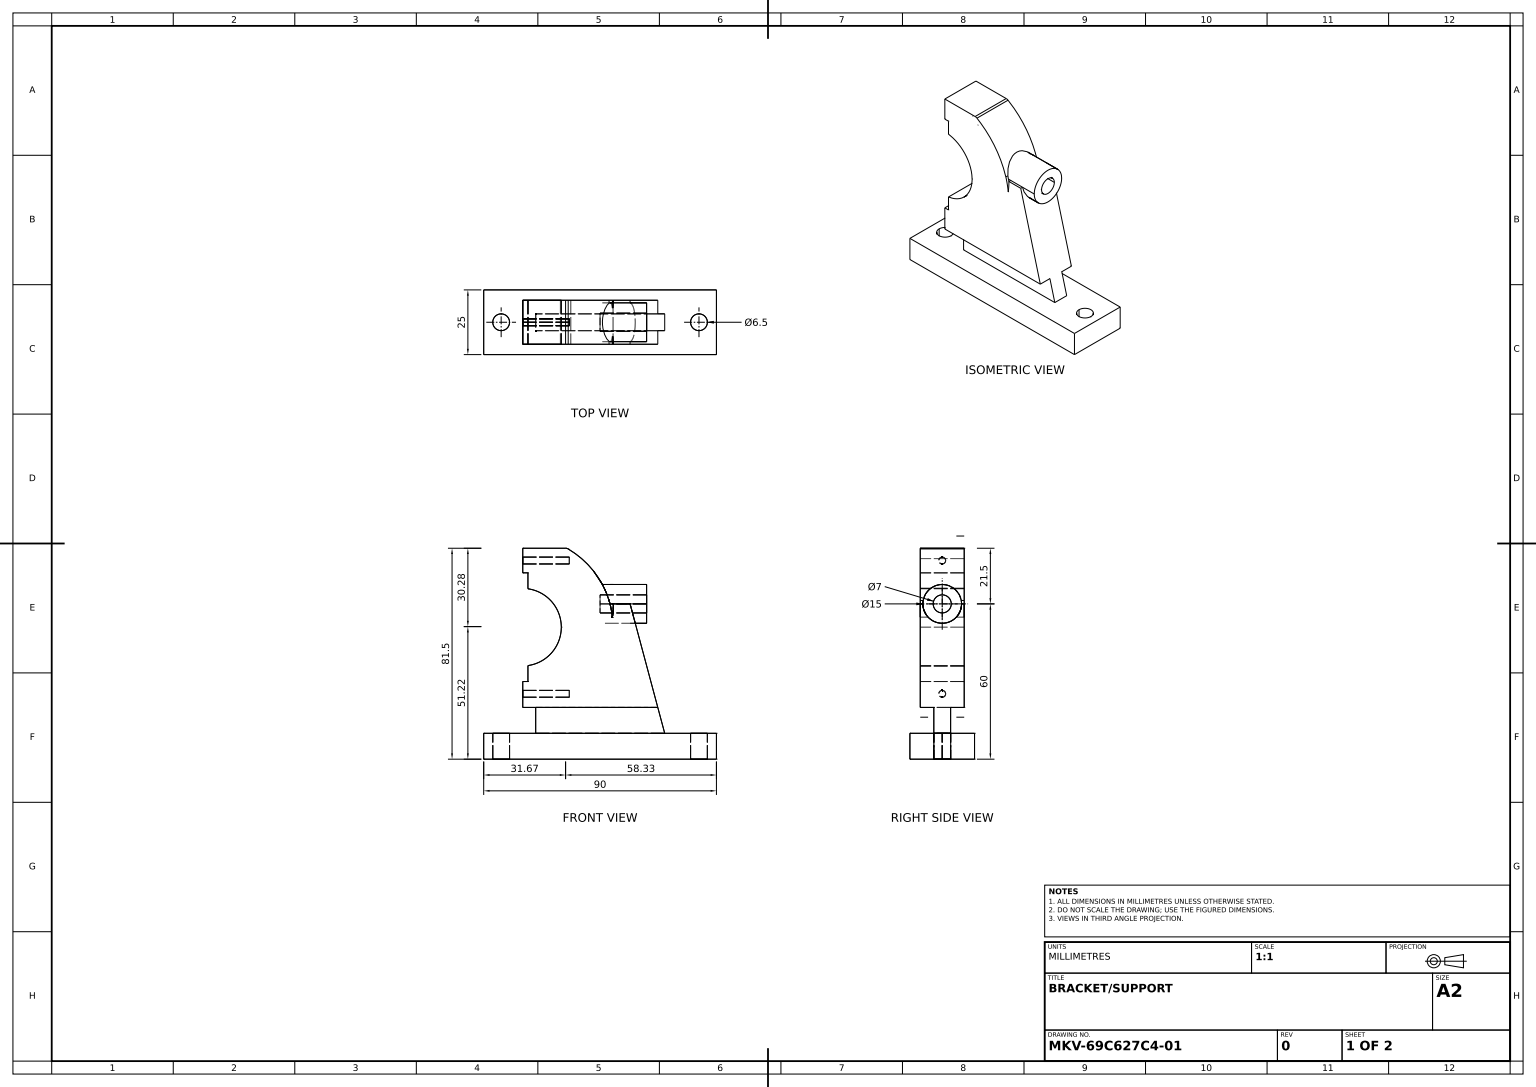
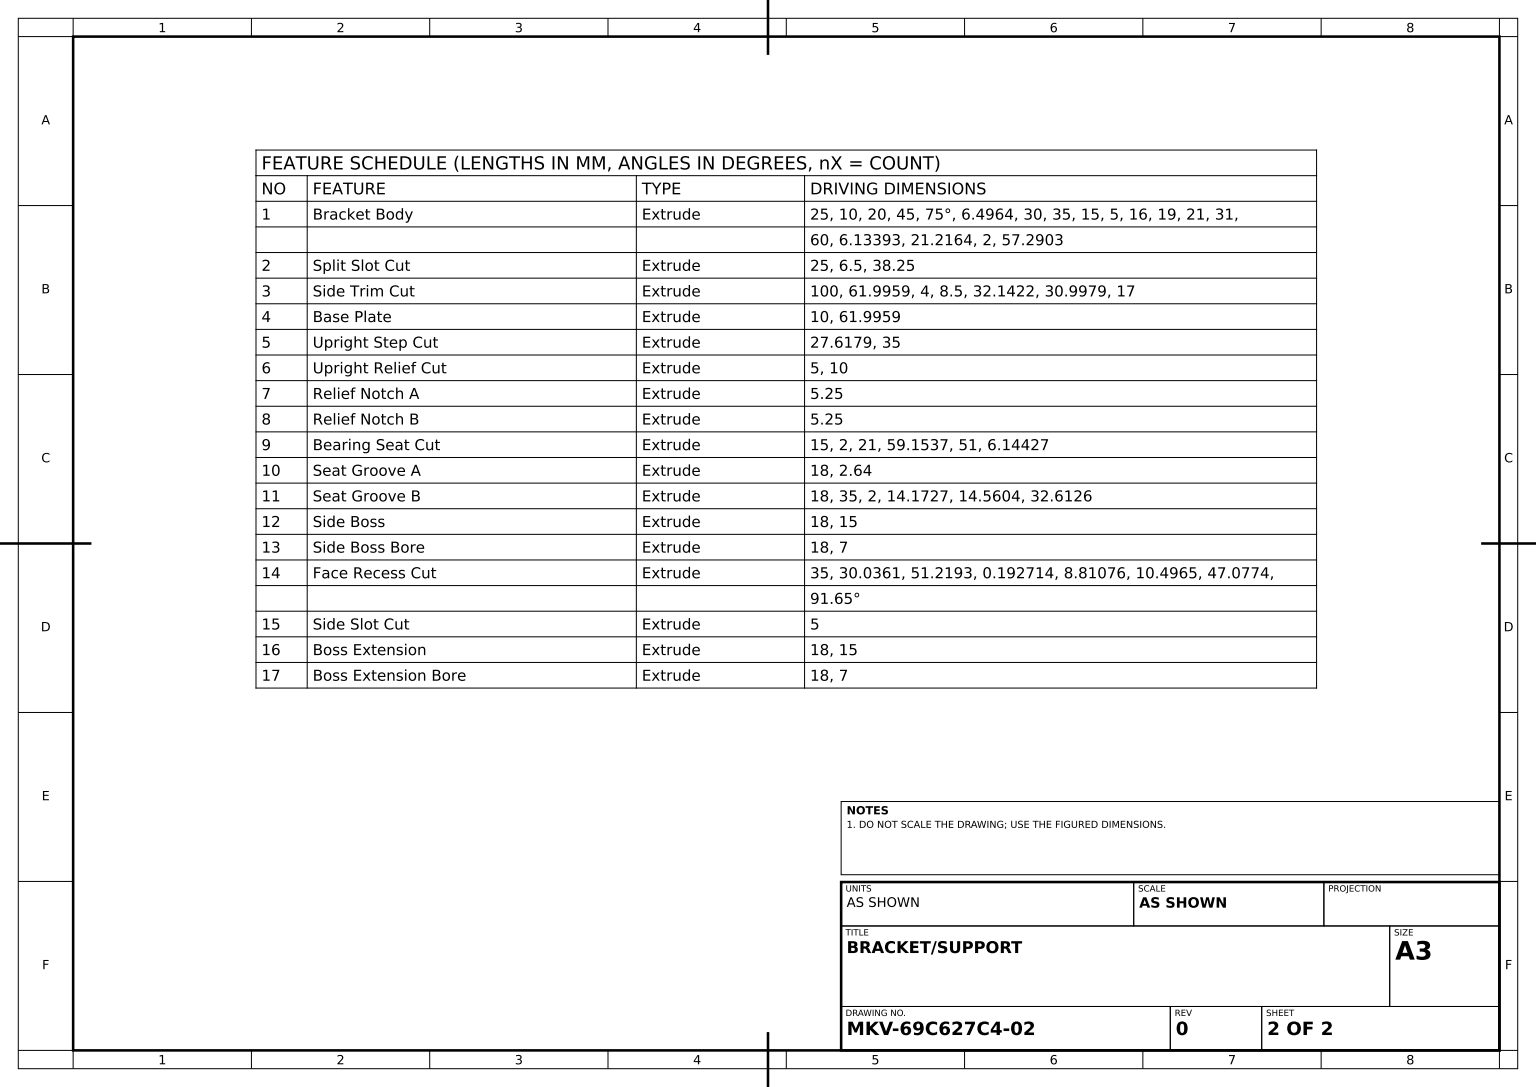
SolidWorks part; units mm, degrees
material "Plain Carbon Steel"
ref_plane "Front Plane" through (0, 0, 0) normal (0, 0, 1) x (1, 0, 0)
ref_plane "Top Plane" through (0, 0, 0) normal (0, 1, 0) x (1, 0, 0)
ref_plane "Right Plane" through (0, 0, 0) normal (1, 0, 0) x (0, 0, -1)
sketch "Bracket Profile Sketch" plane through (0, 0, 0) normal (0, 0, 1) x (1, 0, 0)
  line L0 (0, 0) -> (45, 0)
  line L1 (45, 0) -> (45, 10)
  line L2 (45, 10) -> (-45, 10)
  line L3 (-45, 10) -> (-45, 0)
  line L4 (-45, 0) -> (0, 0)
  line L5 (-45, 10) -> (-29.8939, 10) construction
  line L6 (-29.8939, 10) -> (-29.8939, 29)
  line L7 (-29.8939, 10) -> (-24.8939, 10)
  line L8 (-24.8939, 10) -> (-24.8939, 20)
  line L9 (-24.8939, 20) -> (-29.8939, 20)
  line L10 (-29.8939, 60) -> (-29.8939, 81)
  line L11 (-29.8939, 81) -> (-27.8939, 81)
  line L12 (-27.8939, 81) -> (-27.8939, 74.8661)
  line L13 (-27.8939, 39) -> (-29.8939, 39)
  line L14 (-27.8939, 45.1339) -> (-27.8939, 39)
  line L15 (-29.8939, 60) -> (-29.8939, 29)
  line L16 (-29.8939, 10) -> (-13.8939, 10)
  line L17 (-13.8939, 10) -> (-13.8939, 91.1288)
  line L18 (-29.8939, 29) -> (-13.8939, 28.8712)
  line L19 (-29.8939, 60) -> (27.3964, 60) construction
  line L20 (-29.8939, 91) -> (-13.8939, 91.1288)
  line L21 (-29.8939, 60) -> (-29.8939, 91)
  line L22 (-29.8939, 81) -> (-29.8939, 79)
  line L23 (-27.8939, 79) -> (-6.6775, 79)
  line L24 (-27.8939, 41) -> (-6.6775, 41)
  line L25 (45, 10) -> (25, 10) construction
  line L26 (25, 10) -> (11.6025, 60) construction
  line L27 (5.1061, 60) -> (11.6025, 60)
  line L28 (11.6025, 60) -> (25, 10)
  arc A0 (-27.8939, 45.1339) -> (-27.8939, 74.8661) centre (-29.8939, 60) ccw
  arc A1 (-13.8939, 28.8712) -> (-13.8939, 91.1288) centre (-29.8939, 60) ccw
  arc A2 (-6.6775, 41) -> (-6.6775, 79) centre (-29.8939, 60) ccw
  dimension "D1" = 10
  dimension "D2" = 20
  dimension "D7" = 30
  dimension "D8" = 35
  dimension "D9" = 15
  dimension "D3" = 45
  dimension "D4" = 10
  dimension "D5" = 75
  dimension "D6" = 6.4964
  dimension "D10" = 5
  dimension "D11" = 16
  dimension "D12" = 19
  dimension "D13" = 21
  dimension "D14" = 31
  dimension "D15" = 45
  dimension "D16" = 60
  dimension "D17" = 6.1339
  dimension "D18" = 21.2164
  dimension "D19" = 2
  dimension "D20" = 21
  dimension "D21" = 57.2903
extrude "Bracket Body" add sketch "Bracket Profile Sketch" along normal mid plane 25 contours L3 L4 L0 L1 L2 | A1 L17 L2 L28 L27 | L18 L6 L9 L8 L2 L17 | L8 L9 L6 L2 | A2 L24 L17 A1 L23 | L24 L14 L13 L15 L18 L17 | A0 L14 L24 L17 L23 L12 | L24 A2 L23 L17 | L14 A0 L12 L11 L21 L10 L15 L13 | L12 L23 L17 L20 L21 L11
sketch "Split Slot Sketch" plane through (0, 10, 0) normal (0, 1, 0) x (1, 0, 0)
  line L0 (-45, 0) -> (-38.25, 0) construction
  line L1 (-45, -12.5) -> (-45, 12.5) construction
  line L2 (0, 0) -> (0, 8.9503) construction
  circle A0 centre (-38.25, 0) radius 3.25
  circle A1 centre (38.25, 0) radius 3.25
  dimension "D1" = 6.5
  dimension "D2" = 38.25
extrude "Split Slot Cut" cut sketch "Split Slot Sketch" against normal blind 25
sketch "Side Trim Sketch" plane through (0, 0, 0) normal (0, 1, 0) x (1, 0, 0)
  line L0 (-30.9979, 8.5) -> (-30.9979, 12.5)
  line L1 (-30.9979, 8.5) -> (30.9979, 8.5)
  line L3 (-30.9979, -8.5) -> (30.9979, -8.5)
  line L7 (-29.8939, 12.5) -> (-45, 12.5) construction
  line L8 (-30.9979, 12.5) -> (30.9979, 12.5)
  line L9 (45, 12.5) -> (25, 12.5) construction
  line L10 (30.9979, 12.5) -> (30.9979, 8.5)
  line L11 (-30.9979, -8.5) -> (-30.9979, -12.5)
  line L12 (-29.8939, -12.5) -> (-45, -12.5) construction
  line L13 (-30.9979, -12.5) -> (30.9979, -12.5)
  line L14 (45, -12.5) -> (25, -12.5) construction
  line L15 (30.9979, -12.5) -> (30.9979, -8.5)
  point P0 (0, 0)
  dimension "D1" = 61.9959
  dimension "D2" = 4
  dimension "D3" = 8.5
  dimension "D4" = 32.1422
  dimension "D5" = 30.9979
  dimension "D6" = 17
extrude "Side Trim Cut" cut sketch "Side Trim Sketch" along normal blind 100
sketch "Base Plate Sketch" plane through (0, 0, 0) normal (0, 1, 0) x (1, 0, 0)
  line L0 (-30.9979, 12.5) -> (30.9979, 12.5)
  line L1 (30.9979, 12.5) -> (30.9979, 8.5)
  line L2 (30.9979, 8.5) -> (-30.9979, 8.5)
  line L3 (-30.9979, 12.5) -> (-30.9979, 8.5) construction
  line L4 (-30.9979, 8.5) -> (-30.9979, 12.5)
  line L5 (-30.9979, -8.5) -> (-30.9979, -12.5)
  line L6 (-30.9979, -12.5) -> (30.9979, -12.5)
  line L7 (30.9979, -12.5) -> (30.9979, -8.5)
  line L8 (30.9979, -8.5) -> (-30.9979, -8.5)
  dimension "D1" = 61.9959
extrude "Base Plate" add sketch "Base Plate Sketch" along normal blind 10
sketch "Upright Step Sketch" plane through (0, 0, 8.5) normal (0, 0, 1) x (1, 0, 0)
  line L2 (-29.8939, 10) -> (-29.8939, 91) construction
  line L3 (-29.8939, 81.5) -> (-2.2759, 81.5)
  line L5 (-29.8939, 81.5) -> (-29.8939, 91)
  line L6 (-29.8939, 91) -> (-13.8939, 91.1288)
  arc A0 (5.1061, 60) -> (-13.8939, 91.1288) centre (-29.8939, 60) ccw construction
  arc A3 (-2.2759, 81.5) -> (-13.8939, 91.1288) centre (-29.8939, 60) ccw
  dimension "D1" = 27.6179
  dimension "D2" = 35
extrude "Upright Step Cut" cut sketch "Upright Step Sketch" against normal through all
sketch "Upright Relief Sketch" plane through (0, 0, 8.5) normal (0, 0, 1) x (1, 0, 0)
  line L0 (-29.8939, 10) -> (-24.8939, 10)
  line L1 (45, 10) -> (-45, 10) construction
  line L2 (-24.8939, 10) -> (-24.8939, 20)
  line L3 (-24.8939, 20) -> (-29.8939, 20)
  line L4 (-29.8939, 10) -> (-29.8939, 81.5) construction
  line L5 (-29.8939, 20) -> (-29.8939, 10)
  line L6 (25, 10) -> (-29.8939, 10) construction
  dimension "D1" = 5
  dimension "D2" = 10
extrude "Upright Relief Cut" cut sketch "Upright Relief Sketch" against normal through all
sketch "Relief Notch A Sketch" plane through (-24.8939, 0, 0) normal (-1, 0, 0) x (0, 0, 1)
  line L0 (0, 10) -> (3.25, 10)
  line L1 (-8.5, 10) -> (8.5, 10) construction
  line L2 (3.25, 10) -> (3.25, 20)
  line L3 (-8.5, 20) -> (8.5, 20) construction
  line L4 (3.25, 20) -> (8.5, 20)
  line L5 (8.5, 20) -> (8.5, 10)
  line L6 (12.5, 10) -> (-12.5, 10) construction
  line L7 (8.5, 10) -> (3.25, 10)
  line M3 (-8.5, 10) -> (8.5, 10)
  line M4 (8.5, 10) -> (8.5, 20)
  line M5 (8.5, 20) -> (-8.5, 20)
  dimension "D1" = 5.25
extrude "Relief Notch A" cut sketch "Relief Notch A Sketch" against normal through all contours L2 M3 M4 M5
sketch "Relief Notch B Sketch" plane through (-24.8939, 0, 0) normal (-1, 0, 0) x (0, 0, 1)
  line L0 (0, 10) -> (-3.25, 10)
  line L2 (12.5, 10) -> (-12.5, 10) construction
  line L3 (-3.25, 10) -> (-3.25, 20)
  line L4 (-8.5, 20) -> (3.25, 20) construction
  line L5 (-3.25, 20) -> (-8.5, 20)
  line L6 (-8.5, 20) -> (-8.5, 10)
  line L7 (-8.5, 10) -> (-3.25, 10)
  line M3 (3.25, 20) -> (-8.5, 20)
  line M4 (-8.5, 20) -> (-8.5, 10)
  line M5 (-8.5, 10) -> (3.25, 10)
  dimension "D1" = 5.25
extrude "Relief Notch B" cut sketch "Relief Notch B Sketch" against normal through all contours L3 M5 M3 M4
sketch "Bearing Seat Sketch" plane through (0, 0, 8.5) normal (0, 0, 1) x (1, 0, 0)
  line L0 (-45, 0) -> (-45, 51) construction
  line L1 (-45, 51) -> (-44.9692, 51) construction
  line L3 (-29.8939, 32.8604) -> (-29.8939, 82.8604) construction
  line L4 (-29.8939, 20) -> (-29.8939, 81.5) construction
  line L5 (-29.9692, 51) -> (-29.8939, 30)
  line L6 (-29.8939, 30) -> (-27.8939, 30)
  line L7 (-27.8939, 30) -> (-27.8939, 36.1443)
  line L8 (-29.9692, 51) -> (-3.7789, 51) construction
  line L9 (-27.8939, 72) -> (-27.8939, 65.8557)
  line L10 (-29.8939, 72) -> (-27.8939, 72)
  line L11 (-29.9692, 51) -> (-29.8939, 72)
  arc A0 (-27.8939, 36.1443) -> (-27.8939, 65.8557) centre (-29.9692, 51) ccw
  dimension "D1" = 15
  dimension "D2" = 2
  dimension "D3" = 21
  dimension "D4" = 59.1537
  dimension "D5" = 51
  dimension "D6" = 6.1443
extrude "Bearing Seat Cut" cut sketch "Bearing Seat Sketch" against normal through all
sketch "Seat Groove A Sketch" plane through (-29.8939, 0, 0) normal (-1, 0, 0) x (0, 0, 1)
  line L0 (0, 81.5) -> (0, 20) construction
  line L1 (-8.5, 81.5) -> (8.5, 81.5) construction
  line L2 (-8.5, 20) -> (8.5, 20) construction
  line L5 (8.5, 76.75) -> (-8.5, 76.75) construction
  line L6 (8.5, 72) -> (8.5, 81.5) construction
  line L7 (-8.5, 81.5) -> (-8.5, 72) construction
  line L8 (-8.5, 51) -> (8.5, 51) construction
  line L9 (-8.5, 65.8557) -> (-8.5, 36.1443) construction
  line L10 (8.5, 36.1443) -> (8.5, 65.8557) construction
  circle A0 centre (0, 76.75) radius 1.32
  circle A1 centre (0, 25.25) radius 1.32
  dimension "D1" = 2.64
extrude "Seat Groove A" cut sketch "Seat Groove A Sketch" against normal blind 18
sketch "Seat Groove B Sketch" plane through (0, 0, 8.5) normal (0, 0, 1) x (1, 0, 0)
  line L0 (-29.8939, 20) -> (-13.7212, 20)
  line L1 (-13.3334, 81.5) -> (-2.2759, 81.5)
  line L2 (-29.9692, 93.7843) -> (-29.9692, 2.1723) construction
  line L3 (-29.8939, 81.5) -> (-13.3334, 81.5)
  line L4 (-27.8939, 65.8557) -> (-27.8939, 72) construction
  line L5 (-13.3334, 81.5) -> (-2.2759, 81.5)
  arc A0 (4.7188, 55.6629) -> (-2.2759, 81.5) centre (-29.9949, 60.1305) ccw
  arc A2 (-12.3252, 81.2273) -> (-13.3334, 81.5) centre (-13.3334, 79.5) ccw
  arc A4 (-13.7212, 20) -> (-12.3252, 81.2273) centre (-29.9692, 51) ccw
  line M14 (-2.2759, 81.5) -> (-29.8939, 81.5)
  dimension "D1" = 35
  dimension "D2" = 2
  dimension "D3" = 14.1727
  dimension "D4" = 14.5604
  dimension "D5" = 32.6126
extrude "Seat Groove B" cut sketch "Seat Groove B Sketch" against normal blind 18 contours A4 A0 A2 M14
sketch "Side Boss Sketch" plane through (0, 0, 0) normal (1, 0, 0) x (0, 0, -1)
  line L0 (-8.5, 60) -> (8.5, 60) construction
  circle A0 centre (0, 60) radius 7.5
  dimension "D1" = 15
extrude "Side Boss" add sketch "Side Boss Sketch" along normal blind 18
sketch "Side Boss Bore Sketch" plane through (18, 0, 0) normal (1, 0, 0) x (0, 0, -1)
  circle A0 centre (0, 60) radius 3.5
  dimension "D1" = 7
extrude "Side Boss Bore" cut sketch "Side Boss Bore Sketch" against normal blind 18
sketch "Face Recess Sketch" plane through (0, 0, 0) normal (0, 0, 1) x (1, 0, 0)
  line L0 (-30.0361, 51.2193) -> (-28.6816, 98.2773) construction
  line L1 (-30.0361, 51.2193) -> (9.9691, 51.2193) construction
  line L2 (-12.3252, 81.2273) -> (-1.8309, 81.0134)
  arc A3 (4.7734, 54.8654) -> (-12.011, 81.2209) centre (-30.0361, 51.2193) ccw
  arc A4 (4.7734, 54.8654) -> (-1.8309, 81.0134) centre (-29.8434, 60.0301) ccw
  dimension "D1" = 35
  dimension "D2" = 30.0361
  dimension "D3" = 51.2193
  dimension "D4" = 0.1927
  dimension "D5" = 8.8108
  dimension "D6" = 10.4965
  dimension "D7" = 47.0774
  dimension "D8" = 91.649
extrude "Face Recess Cut" cut sketch "Face Recess Sketch" against normal through all both and the other way through all contours A3 A4 L2
sketch "Side Slot Sketch" plane through (0, 0, 0) normal (1, 0, 0) x (0, 0, -1)
  line L0 (-8.5, 81.5) -> (8.5, 81.5)
  line L1 (8.5, 81.5) -> (8.5, 81.2273)
  line L2 (-8.5, 81.5) -> (-8.5, 81.0149)
  line L3 (-8.5, 81.0149) -> (8.5, 81.0149)
  line L4 (8.5, 81.0149) -> (-8.5, 81.0149) construction
  line L5 (8.5, 81.0149) -> (8.5, 81.5)
extrude "Side Slot Cut" cut sketch "Side Slot Sketch" against normal blind 5 contours L3 L5 L1 L0 L2
sketch "Boss Extension Sketch" plane through (18, 0, 0) normal (1, 0, 0) x (0, 0, -1)
  circle A0 centre (0, 60) radius 7.5
  dimension "D1" = 15
extrude "Boss Extension" add sketch "Boss Extension Sketch" against normal blind 18
sketch "Boss Extension Bore Sketch" plane through (18, 0, 0) normal (1, 0, 0) x (0, 0, -1)
  circle A0 centre (0, 60) radius 3.5
  dimension "D1" = 7
extrude "Boss Extension Bore" cut sketch "Boss Extension Bore Sketch" against normal blind 18
